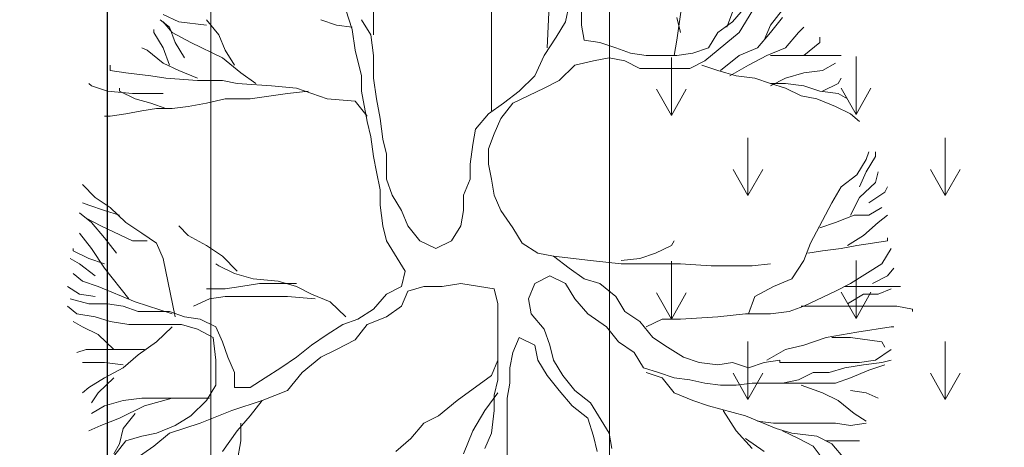
# Model space of a CAD drawing. Units: millimetres. Extents: x 595116 to 630915, y 909473 to 920225.
# Tile 43 of 134: x 629500 to 629559, y 919216 to 919242. Entities that reach past the tile are written whole.
import ezdxf

# ---------------------------------------------------------------- set-up
doc = ezdxf.new("R2010")
doc.units = ezdxf.units.MM
doc.layers.add('Dimension', color=3, linetype='Continuous', lineweight=18)
doc.layers.add('L-PLNT', color=85, linetype='Continuous', lineweight=13)
doc.styles.get("Standard").update_dxf_attribs({"font": 'arial.ttf'})
doc.dimstyles.new('ISO-25', dxfattribs={"dimtxt": 9, "dimasz": 6, "dimexe": 1.25, "dimexo": 0.625, "dimtad": 1, "dimlunit": 4, "dimtxsty": 'Standard', "dimcen": 2.5, "dimadec": 0, "dimazin": 0, "dimtfac": 1, "dimtmove": 0, "dimatfit": 3, "dimfxl": 1, "dimarcsym": 0})

# ---------------------------------------------------------------- blocks, each defined once
blk = doc.blocks.new('A$C143125F4')
for p, q in [((2.5, 3.4584), (2.5, 4.4306)), ((1.8053, 3.9064), (1.8053, 4.2514)), ((3.9607, 3.9199), (4.1248, 4.1887)), ((2.8283, 3.8303), (2.8447, 4.1618)), ((3.5941, 3.8751), (3.6324, 4.1439)), ((2.9377, 3.9826), (2.9596, 4.0856)), ((3.999, 4.0722), (3.9224, 3.9826)), ((0.6565, 3.9826), (0.5635, 4.0274)), ((1.6795, 3.9378), (1.6412, 4.0543)), ((3.0307, 3.9647), (3.0307, 4.0543)), ((3.616, 3.9199), (3.5941, 4.0095)), ((3.8895, 3.9512), (3.9224, 4.0408)), ((4.1467, 3.9647), (4.2178, 4.0543)), ((4.1467, 3.9199), (4.2178, 4.0095)), ((0.6018, 3.9512), (0.5471, 3.996)), ((0.6182, 3.9199), (0.5635, 3.9826)), ((0.6346, 3.8616), (0.6018, 3.9512)), ((0.8206, 3.9647), (0.6565, 3.9826)), ((0.8917, 3.9064), (0.8206, 3.996)), ((1.5865, 3.9647), (1.4935, 3.996)), ((1.6795, 3.9512), (1.5865, 3.9647)), ((1.7342, 3.996), (1.7889, 3.9064)), ((2.883, 3.893), (2.9377, 3.9826)), ((3.0471, 3.8751), (3.0307, 3.9647)), ((3.9224, 3.9826), (3.8348, 3.9199)), ((4.1084, 3.8751), (4.1467, 3.9647)), ((4.3108, 3.9199), (4.3436, 3.9512)), ((0.5088, 3.9199), (0.5088, 3.9378)), ((0.5635, 3.8303), (0.5088, 3.9199)), ((0.7276, 3.8616), (0.6182, 3.9199)), ((0.93, 3.8168), (0.8917, 3.9064)), ((1.6959, 3.8168), (1.6795, 3.9378)), ((1.7889, 3.9064), (1.8053, 3.7855)), ((2.8119, 3.7855), (2.883, 3.893)), ((3.7583, 3.7541), (3.9607, 3.9199)), ((3.8348, 3.9199), (3.7801, 3.8303)), ((4.0701, 3.8303), (4.1467, 3.9199)), ((4.2342, 3.8303), (4.3108, 3.9199)), ((4.4366, 3.8616), (4.4366, 3.893)), ((0.6893, 3.772), (0.6346, 3.8616)), ((0.9136, 3.772), (0.7276, 3.8616)), ((3.1401, 3.8616), (3.0471, 3.8751)), ((3.2331, 3.8303), (3.1401, 3.8616)), ((3.5777, 3.7855), (3.5941, 3.8751)), ((4.3436, 3.7855), (4.4366, 3.8616)), ((0.4705, 3.8168), (0.4376, 3.8303)), ((0.5635, 3.7407), (0.4705, 3.8168)), ((0.6018, 3.7272), (0.5635, 3.8303)), ((0.9847, 3.7272), (0.93, 3.8168)), ((1.7342, 3.6645), (1.6959, 3.8168)), ((1.8053, 3.7855), (1.8053, 3.6511)), ((2.7571, 3.6645), (2.8119, 3.7855)), ((3.3206, 3.7989), (3.2331, 3.8303)), ((3.4136, 3.7855), (3.3206, 3.7989)), ((3.5941, 3.7855), (3.4136, 3.7855)), ((3.6871, 3.7989), (3.5941, 3.7855)), ((3.7801, 3.8303), (3.6871, 3.7989)), ((3.8512, 3.6959), (3.9607, 3.7855)), ((3.9607, 3.7855), (4.0701, 3.8303)), ((4.0154, 3.7272), (4.1248, 3.7855)), ((4.1248, 3.7855), (4.2342, 3.8303)), ((4.1467, 3.7855), (4.5624, 3.7855)), ((0.2516, 3.6959), (0.2516, 3.7272)), ((0.6565, 3.6959), (0.5635, 3.7407)), ((1.023, 3.6824), (0.9136, 3.772)), ((2.8994, 3.6376), (2.9924, 3.7272)), ((2.9924, 3.7272), (3.1018, 3.7541)), ((3.1018, 3.7541), (3.1948, 3.772)), ((3.1948, 3.772), (3.2878, 3.7541)), ((3.2878, 3.7541), (3.3753, 3.7093)), ((3.6707, 3.7093), (3.7583, 3.7541)), ((3.7418, 3.7272), (3.8348, 3.6959)), ((3.906, 3.6645), (4.0154, 3.7272)), ((4.453, 3.6959), (4.5296, 3.7407)), ((0.3446, 3.6824), (0.2516, 3.6959)), ((0.4923, 3.6645), (0.3446, 3.6824)), ((0.5799, 3.6511), (0.4923, 3.6645)), ((0.7659, 3.6511), (0.6565, 3.6959)), ((1.1105, 3.6197), (1.023, 3.6824)), ((1.7342, 3.5749), (1.7342, 3.6645)), ((2.6641, 3.5749), (2.7571, 3.6645)), ((3.3753, 3.7093), (3.6707, 3.7093)), ((3.8348, 3.6959), (3.9442, 3.6645)), ((3.9442, 3.6645), (4.0537, 3.6511)), ((4.2342, 3.6511), (4.3436, 3.6824)), ((4.3436, 3.6824), (4.453, 3.6959)), ((0.1422, 3.6063), (0.1258, 3.6197)), ((0.2352, 3.5749), (0.1422, 3.6063)), ((0.7659, 3.6376), (0.5799, 3.6511)), ((0.9136, 3.6376), (0.7659, 3.6376)), ((1.0011, 3.6197), (0.9136, 3.6376)), ((1.2035, 3.6063), (1.0011, 3.6197)), ((1.3512, 3.5928), (1.2035, 3.6063)), ((1.8053, 3.6511), (1.8217, 3.5301)), ((2.8119, 3.5928), (2.8994, 3.6376)), ((4.0537, 3.6511), (4.1467, 3.6197)), ((4.1467, 3.6063), (4.2342, 3.6511)), ((4.1467, 3.6197), (4.2342, 3.5928)), ((4.1467, 3.6197), (4.2342, 3.6197)), ((4.2342, 3.6197), (4.3436, 3.6063)), ((4.3436, 3.6063), (4.4366, 3.5749)), ((4.453, 3.5749), (4.546, 3.6197)), ((4.546, 3.6197), (4.5624, 3.6511)), ((0.3829, 3.5615), (0.2352, 3.5749)), ((0.3063, 3.5749), (0.3063, 3.5928)), ((0.3993, 3.5301), (0.3063, 3.5749)), ((0.5635, 3.5615), (0.3829, 3.5615)), ((1.2965, 3.5615), (1.0777, 3.5301)), ((1.4223, 3.5749), (1.2965, 3.5615)), ((1.5317, 3.5301), (1.3512, 3.5928)), ((1.767, 3.3957), (1.7342, 3.5749)), ((2.5711, 3.5032), (2.6641, 3.5749)), ((2.6259, 3.5032), (2.8119, 3.5928)), ((4.2342, 3.5928), (4.3272, 3.548)), ((4.3272, 3.548), (4.4202, 3.5301)), ((4.4366, 3.5749), (4.546, 3.5615)), ((4.546, 3.5615), (4.6007, 3.5301)), ((0.4923, 3.5032), (0.3993, 3.5301)), ((0.5799, 3.4719), (0.4923, 3.5032)), ((0.7112, 3.4853), (0.6182, 3.4719)), ((0.8206, 3.5032), (0.7112, 3.4853)), ((0.93, 3.5301), (0.8206, 3.5032)), ((1.0777, 3.5301), (0.93, 3.5301)), ((1.6959, 3.5167), (1.5317, 3.5301)), ((1.767, 3.4271), (1.6959, 3.5167)), ((1.8217, 3.5301), (1.8436, 3.4136)), ((2.4836, 3.4405), (2.5711, 3.5032)), ((2.5547, 3.4136), (2.6259, 3.5032)), ((4.4202, 3.5301), (4.5296, 3.4853)), ((4.5296, 3.4853), (4.6171, 3.4405)), ((0.2516, 3.4271), (0.2188, 3.4271)), ((0.3446, 3.4405), (0.2516, 3.4271)), ((0.4376, 3.4584), (0.3446, 3.4405)), ((0.5252, 3.4719), (0.4376, 3.4584)), ((0.6182, 3.4719), (0.5252, 3.4719)), ((2.407, 3.3509), (2.4836, 3.4405)), ((4.6171, 3.4405), (4.6718, 3.3957)), ((1.7889, 3.3061), (1.767, 3.3957)), ((1.8436, 3.4136), (1.86, 3.2927)), ((2.5164, 3.3241), (2.5547, 3.4136)), ((2.3906, 3.2613), (2.407, 3.3509)), ((2.4836, 3.2345), (2.5164, 3.3241)), ((1.8053, 3.1897), (1.7889, 3.3061)), ((1.86, 3.2927), (1.8819, 3.2031)), ((2.3742, 3.1449), (2.3906, 3.2613)), ((1.8819, 3.2031), (1.8819, 3.0553)), ((2.4836, 3.1449), (2.4836, 3.2345)), ((4.7101, 3.1717), (4.7265, 3.2165)), ((4.7648, 3.1897), (4.7648, 3.2165)), ((1.8217, 3.1001), (1.8053, 3.1897)), ((2.3742, 3.0553), (2.3742, 3.1449)), ((2.5, 3.0553), (2.4836, 3.1449)), ((4.6554, 3.0821), (4.7101, 3.1717)), ((4.7101, 3.1001), (4.7648, 3.1897)), ((1.8436, 2.9925), (1.8217, 3.1001)), ((4.5624, 3.0105), (4.6554, 3.0821)), ((4.6718, 3.0105), (4.7101, 3.1001)), ((4.7648, 3.0373), (4.7812, 3.1001)), ((0.1641, 2.9477), (0.0875, 3.0239)), ((1.8819, 3.0553), (1.9147, 2.9612)), ((2.3359, 2.9612), (2.3742, 3.0553)), ((2.5164, 2.9612), (2.5, 3.0553)), ((4.6718, 2.9477), (4.7648, 3.0373)), ((1.8436, 2.9029), (1.8436, 2.9925)), ((4.5077, 2.9164), (4.5624, 3.0105)), ((4.7265, 2.9164), (4.8195, 2.9791)), ((4.8195, 2.9791), (4.8359, 3.0105)), ((0.1258, 2.9029), (0.0875, 2.9164)), ((0.2516, 2.8895), (0.1641, 2.9477)), ((1.9147, 2.9612), (1.9694, 2.8716)), ((2.3359, 2.8716), (2.3359, 2.9612)), ((2.5547, 2.8716), (2.5164, 2.9612)), ((4.453, 2.8133), (4.5077, 2.9164)), ((4.6171, 2.8447), (4.6718, 2.9477)), ((0.1422, 2.7999), (0.0711, 2.8581)), ((0.1094, 2.8268), (0.0711, 2.8581)), ((0.2188, 2.8716), (0.1258, 2.9029)), ((0.3063, 2.8447), (0.2188, 2.8716)), ((0.3446, 2.7999), (0.2516, 2.8895)), ((1.86, 2.782), (1.8436, 2.9029)), ((1.9694, 2.8716), (2.0077, 2.782)), ((2.3195, 2.782), (2.3359, 2.8716)), ((2.6259, 2.7686), (2.5547, 2.8716)), ((4.7265, 2.8447), (4.8031, 2.8895)), ((0.1969, 2.782), (0.1094, 2.8268)), ((0.2188, 2.7103), (0.1422, 2.7999)), ((0.4376, 2.7372), (0.3446, 2.7999)), ((4.3819, 2.679), (4.453, 2.8133)), ((4.4366, 2.7686), (4.5296, 2.7999)), ((4.5296, 2.7999), (4.639, 2.8447)), ((4.639, 2.8447), (4.7265, 2.8447)), ((4.6937, 2.7238), (4.7812, 2.7999)), ((4.7812, 2.7999), (4.8359, 2.8447)), ((0.1422, 2.6476), (0.0711, 2.7372)), ((0.3829, 2.6924), (0.1969, 2.782)), ((0.5252, 2.679), (0.4376, 2.7372)), ((0.7112, 2.7238), (0.6565, 2.782)), ((1.8819, 2.6924), (1.86, 2.782)), ((2.0077, 2.782), (2.0788, 2.6924)), ((2.2648, 2.6924), (2.3195, 2.782)), ((2.6806, 2.679), (2.6259, 2.7686)), ((0.2899, 2.6207), (0.2188, 2.7103)), ((0.4705, 2.6924), (0.3829, 2.6924)), ((0.5635, 2.5894), (0.5252, 2.679)), ((0.8206, 2.6655), (0.7112, 2.7238)), ((1.9913, 2.5132), (1.8819, 2.6924)), ((2.0788, 2.6924), (2.1718, 2.6476)), ((2.1718, 2.6476), (2.2648, 2.6924)), ((2.7736, 2.6207), (2.6806, 2.679)), ((3.5613, 2.6655), (3.5777, 2.6924)), ((4.3436, 2.5759), (4.3819, 2.679)), ((4.6007, 2.6655), (4.6937, 2.7238)), ((4.6554, 2.6655), (4.7484, 2.679)), ((4.7484, 2.679), (4.8359, 2.6924)), ((4.8359, 2.6924), (4.8359, 2.7103)), ((0.0328, 2.6342), (0.0328, 2.6476)), ((0.1258, 2.5894), (0.0328, 2.6342)), ((0.2188, 2.5311), (0.1422, 2.6476)), ((0.9136, 2.6028), (0.8206, 2.6655)), ((2.8666, 2.6028), (2.7736, 2.6207)), ((3.3753, 2.5894), (3.4683, 2.6207)), ((3.4683, 2.6207), (3.5613, 2.6655)), ((4.3655, 2.6207), (4.453, 2.6342)), ((4.453, 2.6342), (4.5624, 2.6476)), ((4.5624, 2.6476), (4.6554, 2.6655)), ((4.8031, 2.558), (4.8578, 2.6476)), ((0.0711, 2.558), (0.0164, 2.5894)), ((0.1641, 2.4863), (0.0711, 2.558)), ((0.2188, 2.558), (0.1258, 2.5894)), ((0.6346, 2.2444), (0.5635, 2.5894)), ((0.8917, 2.5446), (0.8753, 2.558)), ((1.0011, 2.5132), (0.9136, 2.6028)), ((2.8666, 2.6028), (3.0854, 2.5759)), ((2.9596, 2.5311), (2.8666, 2.6028)), ((3.0854, 2.5759), (3.2659, 2.558)), ((3.2659, 2.5759), (3.3753, 2.5894)), ((3.2659, 2.558), (3.616, 2.558)), ((3.616, 2.558), (3.7965, 2.5446)), ((4.0372, 2.5446), (4.1467, 2.558)), ((4.2725, 2.4684), (4.3436, 2.5759)), ((4.6171, 2.4415), (4.8031, 2.558)), ((0.0875, 2.455), (0.0328, 2.4998)), ((0.3611, 2.3519), (0.2188, 2.5311)), ((0.9847, 2.4998), (0.8917, 2.5446)), ((1.0941, 2.4684), (0.9847, 2.4998)), ((1.9694, 2.4236), (1.9913, 2.5132)), ((3.0471, 2.4684), (2.9596, 2.5311)), ((3.7965, 2.5446), (4.0372, 2.5446)), ((4.8359, 2.4863), (4.8742, 2.5311)), ((0.1805, 2.4236), (0.0875, 2.455)), ((1.1324, 2.4415), (1.023, 2.4236)), ((1.2418, 2.455), (1.0941, 2.4684)), ((1.3512, 2.4415), (1.1324, 2.4415)), ((1.3512, 2.4236), (1.2418, 2.455)), ((2.3195, 2.4415), (2.2101, 2.4236)), ((2.4289, 2.4236), (2.3195, 2.4415)), ((2.7571, 2.4415), (2.7189, 2.3519)), ((2.8447, 2.4863), (2.7571, 2.4415)), ((2.9377, 2.4415), (2.8447, 2.4863)), ((2.9924, 2.3519), (2.9377, 2.4415)), ((3.1401, 2.4415), (3.0471, 2.4684)), ((3.2331, 2.3654), (3.1401, 2.4415)), ((4.1631, 2.4236), (4.2725, 2.4684)), ((4.5296, 2.3967), (4.6171, 2.4415)), ((4.7484, 2.4415), (4.8359, 2.4863)), ((0.0711, 2.3788), (0, 2.4236)), ((0.3993, 2.334), (0.1805, 2.4236)), ((0.93, 2.4102), (0.8206, 2.4102)), ((1.023, 2.4236), (0.93, 2.4102)), ((1.4387, 2.3788), (1.3512, 2.4236)), ((1.8819, 2.3788), (1.9694, 2.4236)), ((2.0077, 2.3967), (1.9694, 2.3071)), ((2.1007, 2.4236), (2.0077, 2.3967)), ((2.2101, 2.4236), (2.1007, 2.4236)), ((2.5164, 2.4102), (2.4289, 2.4236)), ((2.5383, 2.3206), (2.5164, 2.4102)), ((4.0537, 2.3654), (4.1631, 2.4236)), ((4.3436, 2.3071), (4.5296, 2.3967)), ((4.5843, 2.4236), (4.9125, 2.4236)), ((4.7812, 2.3788), (4.8578, 2.4102)), ((0.0164, 2.3519), (0.1258, 2.3206)), ((0.1641, 2.3654), (0.0711, 2.3788)), ((0.6182, 2.2623), (0.3993, 2.334)), ((0.837, 2.3519), (0.744, 2.3071)), ((0.93, 2.3654), (0.837, 2.3519)), ((1.2965, 2.3654), (0.93, 2.3654)), ((1.4606, 2.3519), (1.2965, 2.3654)), ((1.5482, 2.334), (1.4387, 2.3788)), ((1.6412, 2.2444), (1.5482, 2.334)), ((1.8053, 2.2892), (1.8819, 2.3788)), ((2.7189, 2.3519), (2.7353, 2.2623)), ((3.069, 2.2623), (2.9924, 2.3519)), ((3.2878, 2.2758), (3.2331, 2.3654)), ((4.0154, 2.2623), (4.0537, 2.3654)), ((4.6007, 2.3206), (4.6937, 2.3788)), ((4.6937, 2.3788), (4.7812, 2.3788)), ((0.0547, 2.2623), (0, 2.3071)), ((0.1258, 2.3206), (0.2352, 2.3206)), ((0.2352, 2.3206), (0.3282, 2.3071)), ((0.3282, 2.3071), (0.4158, 2.2758)), ((0.4158, 2.2758), (0.6018, 2.2758)), ((0.6018, 2.2758), (0.6893, 2.2444)), ((1.7123, 2.231), (1.8053, 2.2892)), ((1.9694, 2.3071), (1.8819, 2.2444)), ((2.5383, 1.8726), (2.5383, 2.3206)), ((3.3753, 2.2175), (3.2878, 2.2758)), ((4.1467, 2.2623), (4.2561, 2.2758)), ((4.2561, 2.2758), (4.3436, 2.3071)), ((4.3272, 2.3071), (4.8906, 2.3071)), ((4.8906, 2.3071), (4.9836, 2.2892)), ((4.9836, 2.2892), (4.9836, 2.2758)), ((0.0875, 2.1862), (0.0328, 2.2175)), ((0.1641, 2.2444), (0.0547, 2.2623)), ((0.2516, 2.2175), (0.1641, 2.2444)), ((0.3611, 2.1996), (0.2516, 2.2175)), ((0.6893, 2.2444), (0.7823, 2.231)), ((0.7823, 2.231), (0.8753, 2.1862)), ((1.6247, 2.1996), (1.7123, 2.231)), ((1.8819, 2.2444), (1.767, 2.1996)), ((2.7353, 2.2623), (2.8119, 2.1727)), ((3.1784, 2.1862), (3.069, 2.2623)), ((3.4519, 2.1235), (3.3753, 2.2175)), ((3.4136, 2.1862), (3.5066, 2.231)), ((3.5066, 2.231), (3.616, 2.231)), ((3.616, 2.231), (3.8348, 2.2444)), ((3.8348, 2.2444), (3.999, 2.2623)), ((3.999, 2.2623), (4.1467, 2.2623)), ((0.1805, 2.1414), (0.0875, 2.1862)), ((0.6729, 2.1996), (0.3611, 2.1996)), ((0.6182, 2.1862), (0.5252, 2.0966)), ((0.7659, 2.1727), (0.6729, 2.1996)), ((0.8589, 2.1235), (0.7659, 2.1727)), ((0.8753, 2.1862), (0.9136, 2.0966)), ((1.5317, 2.1414), (1.6247, 2.1996)), ((1.767, 2.1996), (1.6959, 2.11)), ((2.8119, 2.1727), (2.8447, 2.0787)), ((3.2495, 2.0966), (3.1784, 2.1862)), ((4.4749, 2.1235), (4.6554, 2.1548)), ((4.6554, 2.1548), (4.8578, 2.1862)), ((4.8578, 2.1862), (4.8742, 2.1862)), ((0.2735, 2.0518), (0.1805, 2.1414)), ((0.5252, 2.0966), (0.4158, 2.0204)), ((0.8753, 1.9891), (0.8589, 2.1235)), ((0.9136, 2.0966), (0.9464, 2.007)), ((1.4387, 2.0787), (1.5317, 2.1414)), ((1.6959, 2.11), (1.5865, 2.0518)), ((2.6641, 2.1235), (2.6259, 2.0339)), ((2.7571, 2.0787), (2.6641, 2.1235)), ((3.3425, 2.0339), (3.2495, 2.0966)), ((3.5394, 2.0652), (3.4519, 2.1235)), ((4.3436, 2.0787), (4.4749, 2.1235)), ((4.5077, 2.1235), (4.6171, 2.1235)), ((4.6171, 2.1235), (4.8031, 2.0966)), ((4.8031, 2.0966), (4.8195, 2.0652)), ((0.1094, 2.0518), (0.0547, 2.0339)), ((0.4541, 2.0518), (0.1094, 2.0518)), ((1.3512, 2.007), (1.4387, 2.0787)), ((1.5865, 2.0518), (1.4935, 2.007)), ((2.6259, 2.0339), (2.6094, 1.9443)), ((2.7736, 1.9891), (2.7571, 2.0787)), ((2.8447, 2.0787), (2.8666, 1.9891)), ((3.3972, 1.9443), (3.3425, 2.0339)), ((3.6324, 2.007), (3.5394, 2.0652)), ((4.1248, 1.9891), (4.2342, 2.0518)), ((4.2342, 2.0518), (4.3436, 2.0787)), ((4.8578, 2.0518), (4.7648, 1.9891)), ((0.2188, 1.9756), (0.0875, 1.9756)), ((0.3282, 1.9622), (0.2188, 1.9756)), ((0.4158, 2.0204), (0.3282, 1.9443)), ((0.8753, 1.8412), (0.8753, 1.9891)), ((0.9464, 2.007), (0.9847, 1.9174)), ((1.2582, 1.9443), (1.3512, 2.007)), ((1.4935, 2.007), (1.384, 1.9174)), ((2.5383, 1.9891), (2.5, 1.8995)), ((2.8283, 1.8995), (2.7736, 1.9891)), ((2.8666, 1.9891), (2.9213, 1.8995)), ((3.7254, 1.9756), (3.6324, 2.007)), ((3.8348, 1.9622), (3.7254, 1.9756)), ((3.9224, 1.9756), (3.8348, 1.9622)), ((4.0154, 1.9443), (3.9224, 1.9756)), ((4.1084, 1.9756), (4.0154, 1.9443)), ((4.2014, 1.9891), (4.1084, 1.9756)), ((4.2014, 1.9756), (4.2014, 1.9891)), ((4.6718, 1.9756), (4.2014, 1.9756)), ((4.7648, 1.9891), (4.6718, 1.9756)), ((4.6937, 1.9622), (4.8031, 1.9756)), ((4.8031, 1.9756), (4.8578, 1.9891)), ((0.3282, 1.9443), (0.2188, 1.886)), ((0.9847, 1.9174), (0.9847, 1.8278)), ((1.1652, 1.886), (1.2582, 1.9443)), ((1.384, 1.9174), (1.2965, 1.8099)), ((2.6094, 1.9443), (2.6094, 1.8547)), ((3.4847, 1.9174), (3.3972, 1.9443)), ((3.4136, 1.9174), (3.5066, 1.886)), ((3.5777, 1.886), (3.4847, 1.9174)), ((4.3108, 1.8726), (4.3983, 1.9174)), ((4.3983, 1.9174), (4.4913, 1.9174)), ((4.4913, 1.9174), (4.5843, 1.9443)), ((4.5843, 1.9443), (4.6937, 1.9622)), ((4.7265, 1.9308), (4.6171, 1.886)), ((4.8195, 1.9622), (4.7265, 1.9308)), ((0.2188, 1.886), (0.1258, 1.8278)), ((0.2735, 1.886), (0.1805, 1.7964)), ((1.0777, 1.8278), (1.1652, 1.886)), ((2.5, 1.8995), (2.2976, 1.7516)), ((2.5164, 1.783), (2.5383, 1.8726)), ((2.8994, 1.8099), (2.8283, 1.8995)), ((2.9213, 1.8995), (2.9924, 1.8099)), ((3.5066, 1.886), (3.5777, 1.7964)), ((3.6707, 1.8726), (3.5777, 1.886)), ((3.7583, 1.8547), (3.6707, 1.8726)), ((4.2178, 1.8547), (4.3108, 1.8726)), ((4.6171, 1.886), (4.5296, 1.8547)), ((0.1258, 1.8278), (0.0875, 1.7964)), ((0.8206, 1.7516), (0.8753, 1.8412)), ((0.9847, 1.8278), (1.0777, 1.8278)), ((1.2965, 1.8099), (1.1488, 1.7516)), ((2.6094, 1.8547), (2.593, 1.7651)), ((2.976, 1.7203), (2.8994, 1.8099)), ((2.9924, 1.8099), (3.0854, 1.7382)), ((3.8512, 1.8412), (3.7583, 1.8547)), ((3.9442, 1.8412), (3.8512, 1.8412)), ((4.0372, 1.8547), (3.9442, 1.8412)), ((4.1248, 1.8547), (4.0372, 1.8547)), ((4.5296, 1.8547), (4.1248, 1.8547)), ((4.3272, 1.8412), (4.453, 1.7964)), ((4.6171, 1.8099), (4.7101, 1.7964)), ((0.1805, 1.7964), (0.1422, 1.7382)), ((0.3282, 1.7516), (0.2188, 1.7203)), ((0.4376, 1.7651), (0.3282, 1.7516)), ((0.837, 1.7651), (0.4376, 1.7651)), ((0.6182, 1.7651), (0.4541, 1.7203)), ((0.7276, 1.662), (0.8206, 1.7516)), ((1.1488, 1.7516), (0.9683, 1.6934)), ((1.1488, 1.7516), (1.0777, 1.662)), ((2.2976, 1.7516), (2.1882, 1.662)), ((2.5383, 1.7964), (2.4617, 1.6934)), ((2.5164, 1.6934), (2.5164, 1.783)), ((2.593, 1.7651), (2.593, 1.3932)), ((3.5777, 1.7964), (3.6871, 1.7516)), ((3.6871, 1.7516), (3.7801, 1.7203)), ((4.453, 1.7964), (4.546, 1.7516)), ((4.546, 1.7516), (4.639, 1.6755)), ((4.7101, 1.7964), (4.7812, 1.7651)), ((0.2188, 1.7203), (0.1422, 1.6755)), ((0.4541, 1.7203), (0.3063, 1.6486)), ((0.9683, 1.6934), (0.7823, 1.6172)), ((2.4617, 1.6934), (2.3906, 1.5724)), ((2.5, 1.559), (2.5164, 1.6934)), ((3.069, 1.6486), (2.976, 1.7203)), ((3.0854, 1.7382), (3.1948, 1.559)), ((3.7801, 1.7203), (3.999, 1.662)), ((3.8677, 1.6934), (3.9442, 1.5724)), ((0.3063, 1.6486), (0.1969, 1.6038)), ((0.3993, 1.6755), (0.3282, 1.5859)), ((0.6346, 1.6038), (0.7276, 1.662)), ((1.0777, 1.662), (1.0011, 1.5724)), ((2.1882, 1.662), (2.1007, 1.6172)), ((3.1018, 1.5411), (3.069, 1.6486)), ((3.999, 1.662), (4.1795, 1.5859)), ((4.0701, 1.6307), (4.1631, 1.6172)), ((4.639, 1.6755), (4.7101, 1.6307)), ((0.1969, 1.6038), (0.1258, 1.5724)), ((0.3282, 1.5859), (0.3063, 1.4963)), ((0.5252, 1.559), (0.6346, 1.6038)), ((0.7823, 1.6172), (0.6018, 1.559)), ((1.0011, 1.5724), (0.9136, 1.4515)), ((1.023, 1.6172), (1.023, 1.5142)), ((2.1007, 1.6172), (2.0241, 1.5276)), ((2.3906, 1.5724), (2.3359, 1.438)), ((3.9442, 1.5724), (4.0372, 1.4694)), ((4.1631, 1.6172), (4.5296, 1.6172)), ((4.1795, 1.5859), (4.2725, 1.559)), ((4.2178, 1.5724), (4.3108, 1.5276)), ((4.5296, 1.6172), (4.6171, 1.6038)), ((4.6171, 1.6038), (4.7101, 1.6172)), ((0.2735, 1.4246), (0.3446, 1.5142)), ((0.3446, 1.5142), (0.4376, 1.5411)), ((0.4376, 1.5411), (0.5252, 1.559)), ((0.6018, 1.559), (0.5088, 1.4828)), ((1.023, 1.5142), (1.0011, 1.3932)), ((2.0241, 1.5276), (1.9366, 1.4515)), ((2.4617, 1.4694), (2.5, 1.559)), ((3.1237, 1.4515), (3.1018, 1.5411)), ((3.1948, 1.559), (3.2112, 1.4694)), ((3.999, 1.5276), (4.1084, 1.4515)), ((4.2725, 1.559), (4.4202, 1.5411)), ((4.3108, 1.5276), (4.3983, 1.4828)), ((4.4202, 1.5411), (4.5077, 1.4963)), ((4.4749, 1.5142), (4.6718, 1.5142)), ((0.3063, 1.4963), (0.2735, 1.438)), ((0.5088, 1.4828), (0.3993, 1.4067)), ((4.3983, 1.4828), (4.4749, 1.3798)), ((4.5077, 1.4963), (4.5843, 1.4067))]:
    blk.add_line(p, q)
blk = doc.blocks.new('LAWN-GRASS-TUFT')
blk.add_line((0.892, 3.485), (0.892, 0))
blk.add_lwpolyline([(0, 1.577), (0.892, 0), (1.785, 1.577)])
blk = doc.blocks.new('*D215')
at = {"layer": 'Defpoints', "color": 0, "transparency": 16777216}
for p in [(629316.041, 919411.828), (629505.041, 919411.828), (629505.041, 918832.378)]:
    blk.add_point(p, dxfattribs=at)
at = {"layer": 'Dimension', "color": 0, "lineweight": -2, "transparency": 16777216}
for p, q in [((629316.041, 919411.203), (629316.041, 918831.128)), ((629505.041, 919411.203), (629505.041, 918831.128)), ((629322.041, 918832.378), (629499.041, 918832.378))]:
    blk.add_line(p, q, dxfattribs=at)
at = {"layer": 'Dimension', "color": 0, "transparency": 16777216}
for points in [[(629322.041, 918833.378), (629322.041, 918831.378), (629316.041, 918832.378)], [(629499.041, 918833.378), (629499.041, 918831.378), (629505.041, 918832.378)]]:
    blk.add_solid(points, dxfattribs=at)
at = {"layer": 'Dimension', "color": 0, "transparency": 16777216, "insert": (629410.541, 918837.598), "char_height": 9, "attachment_point": 5}
blk.add_mtext('15\'-9"', dxfattribs=at)
blk = doc.blocks.new('*D216')
at = {"layer": 'Defpoints', "color": 0, "transparency": 16777216}
for p in [(629505.041, 919411.828), (629743.541, 919411.928), (629743.541, 918832.378)]:
    blk.add_point(p, dxfattribs=at)
at = {"layer": 'Dimension', "color": 0, "lineweight": -2, "transparency": 16777216}
for p, q in [((629505.041, 919411.203), (629505.041, 918831.128)), ((629743.541, 919411.303), (629743.541, 918831.128)), ((629511.041, 918832.378), (629737.541, 918832.378))]:
    blk.add_line(p, q, dxfattribs=at)
at = {"layer": 'Dimension', "color": 0, "transparency": 16777216}
for points in [[(629511.041, 918833.378), (629511.041, 918831.378), (629505.041, 918832.378)], [(629737.541, 918833.378), (629737.541, 918831.378), (629743.541, 918832.378)]]:
    blk.add_solid(points, dxfattribs=at)
at = {"layer": 'Dimension', "color": 0, "transparency": 16777216, "insert": (629624.291, 918837.656), "char_height": 9, "attachment_point": 5}
blk.add_mtext('19\'-10 1/2"', dxfattribs=at)
blk = doc.blocks.new('*D221')
at = {"layer": 'Defpoints', "color": 0, "transparency": 16777216}
for p in [(629511.274, 919302.009), (629155.382, 919160.917), (629511.274, 919160.917)]:
    blk.add_point(p, dxfattribs=at)
at = {"layer": 'Dimension', "color": 0, "lineweight": -2, "transparency": 16777216}
for p, q in [((629510.649, 919302.009), (629154.132, 919302.009)), ((629155.382, 919296.009), (629155.382, 919166.917)), ((629510.649, 919160.917), (629154.132, 919160.917))]:
    blk.add_line(p, q, dxfattribs=at)
at = {"layer": 'Dimension', "color": 0, "transparency": 16777216}
for points in [[(629154.382, 919296.009), (629156.382, 919296.009), (629155.382, 919302.009)], [(629154.382, 919166.917), (629156.382, 919166.917), (629155.382, 919160.917)]]:
    blk.add_solid(points, dxfattribs=at)
at = {"layer": 'Dimension', "color": 0, "transparency": 16777216, "insert": (629150.162, 919231.463), "char_height": 9, "attachment_point": 5, "rotation": 90}
blk.add_mtext('11\'-9"', dxfattribs=at)

msp = doc.modelspace()

# ---------------------------------------------------------------- linework, layer by layer
at = {"layer": 'L-PLNT'}
for p, q in [((629511.274, 919302.009), (629511.274, 919160.917)), ((629535.274, 919266.009), (629535.274, 919184.917))]:
    msp.add_line(p, q, dxfattribs=at)

# ---------------------------------------------------------------- block references
at = {"layer": 'L-PLNT', "xscale": 10.20167662382051, "yscale": 10.20167662382051, "zscale": 10.20167662382051}
msp.add_blockref('A$C143125F4', (629502.654, 919201.332), dxfattribs=at)
at = {"layer": 'L-PLNT'}
for p in [(629538.093, 919236.348), (629549.207, 919236.398), (629542.7, 919231.52), (629554.573, 919231.52), (629538.093, 919224.092), (629549.207, 919224.142), (629542.7, 919219.264), (629554.573, 919219.264)]:
    msp.add_blockref('LAWN-GRASS-TUFT', p, dxfattribs=at)

# ---------------------------------------------------------------- dimensions: what is measured, and where the dimension line sits
at = {"layer": 'Dimension'}
for base, p1, p2, picture, middle in [((629505.041, 918832.378), (629316.041, 919411.828), (629505.041, 919411.828), '*D215', (629410.541, 918837.598)), ((629743.541, 918832.378), (629505.041, 919411.828), (629743.541, 919411.928), '*D216', (629624.291, 918837.656))]:
    dim = msp.add_linear_dim(base=base, p1=p1, p2=p2, dimstyle='ISO-25', override={"dimdec": 1, "dimlfac": 1, "dimrnd": 0, "dimzin": 1, "dimdsep": 46, "dimlunit": 4, "dimfrac": 2}, dxfattribs=at)
    dim.commit()
    dim.dimension.update_dxf_attribs({"geometry": picture, "text_midpoint": middle})
dim = msp.add_linear_dim(base=(629155.382, 919160.917), p1=(629511.274, 919302.009), p2=(629511.274, 919160.917), angle=90, dimstyle='ISO-25', override={"dimdec": 1, "dimlfac": 1, "dimrnd": 0, "dimzin": 1, "dimdsep": 46, "dimlunit": 4, "dimfrac": 2}, dxfattribs=at)
dim.commit()
dim.dimension.update_dxf_attribs({"geometry": '*D221', "text_midpoint": (629150.162, 919231.463)})

doc.saveas('drawing.dxf')
